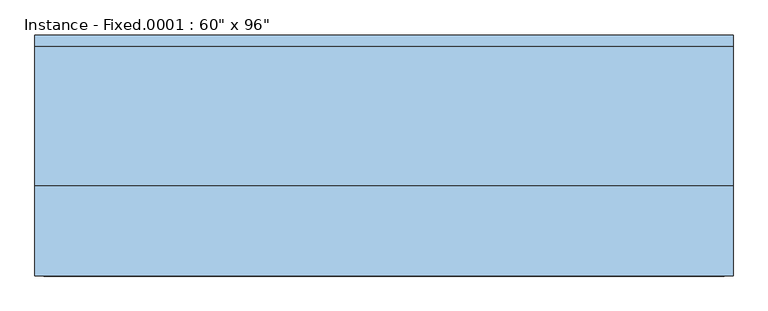
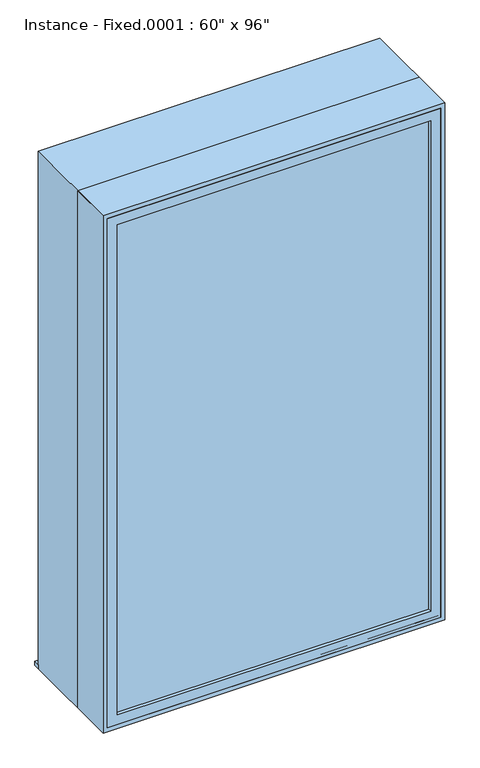
"""IFC4 building model written with IfcOpenShell, lengths in millimetres: window geometry."""

from ifc_helpers import new_model, si_unit, frame, origin, place, context, project, spatial, polyline, outline, extrude, source, transform, mapped, element, save


def window_e9f06afb(model_context):
    return source(origin(), model_context, "Body", "SweptSolid", [
        extrude(outline(polyline([(-800.1, 177.8), (723.9, 177.8), (723.9, 152.4), (-800.1, 152.4), (-800.1, 177.8)])), frame((0.0, 0.0, 609.6), z_axis=(0.0, 0.0, 1.0), x_axis=(1.0, 0.0, 0.0)), (0.0, 0.0, 1.0), 19.05),
        extrude(outline(polyline([(660.4, -333.375), (-736.6, -333.375), (-736.6, -320.675), (660.4, -320.675), (660.4, -333.375)])), frame((0.0, 0.0, 673.1), z_axis=(0.0, 0.0, 1.0), x_axis=(1.0, 0.0, 0.0)), (0.0, 0.0, 1.0), 2311.4),
        extrude(outline(polyline([(3028.95, -781.05), (628.65, -781.05), (628.65, 704.85), (3028.95, 704.85), (3028.95, -781.05)]), holes=[polyline([(2984.5, -736.6), (2984.5, 660.4), (673.1, 660.4), (673.1, -736.6), (2984.5, -736.6)])]), frame((0.0, -349.25, 0.0), z_axis=(0.0, 1.0, 0.0), x_axis=(0.0, 0.0, 1.0)), (0.0, 0.0, 1.0), 44.45),
        extrude(outline(polyline([(3048.0, -800.1), (609.6, -800.1), (609.6, 723.9), (3048.0, 723.9), (3048.0, -800.1)]), holes=[polyline([(3016.25, -768.35), (3016.25, 692.15), (641.35, 692.15), (641.35, -768.35), (3016.25, -768.35)])]), frame((0.0, -349.25, 0.0), z_axis=(0.0, 1.0, 0.0), x_axis=(0.0, 0.0, 1.0)), (0.0, 0.0, 1.0), 196.85),
        extrude(outline(polyline([(3048.0, 723.9), (3048.0, -800.1), (609.6, -800.1), (609.6, 723.9), (3048.0, 723.9)]), holes=[polyline([(3028.95, 704.85), (628.65, 704.85), (628.65, -781.05), (3028.95, -781.05), (3028.95, 704.85)])]), frame((0.0, -349.25, 0.0), z_axis=(0.0, 1.0, 0.0), x_axis=(0.0, 0.0, 1.0)), (0.0, 0.0, 1.0), 501.65),
    ])


if __name__ == "__main__":
    model = new_model("IFC4")
    model_context = context("Model", 3, world=origin())
    ifc_project = project(units=[si_unit("LENGTHUNIT", "METRE", prefix="MILLI")], contexts=[model_context])
    site = spatial("IfcSite", under=ifc_project)
    building = spatial("IfcBuilding", under=site)
    placement = place(None, origin())
    window_shape = window_e9f06afb(model_context)
    element("IfcWindow", 1, ObjectType="Instance - Fixed.0001 : 60\" x 96\"", at=placement, inside=building, context=model_context, shape_type="MappedRepresentation", body=[
        mapped(window_shape, transform((0.0, 0.0, 0.0), x_axis=(1.0, 0.0, 0.0), y_axis=(0.0, 1.0, 0.0), z_axis=(0.0, 0.0, 1.0))),
    ])
    save(model, "model.ifc")

# Revit data of these elements
# Type "Instance - Fixed.0001 : 60\" x 96\""
#   Type Mark = "13"
#   Construction Type Id = "MDOOR"
#   Assembly Code = "B2020100"
#   Analytic Construction = "Metal"
#   Heat Transfer Coefficient (U) = 0.651978 BTU/(h·ft²·°F)
#   Height [instance default] = 6' - 0"
#   Default Sill Height = 2' - 0"
#   Width [instance default] = 3' - 0"
#   Window Inset = 1' - 6"
#   Define Thermal Properties by = 1
#   Glass Pane Material = Glass
#   Sash Material = Door - Frame
#   Visual Light Transmittance = 0
#   Thermal Resistance (R) = 0
#   Solar Heat Gain Coefficient = 0
#   Wall Closure = (empty or 0)
# Element 1 (IfcWindow, "Instance - Fixed.0001 : 60\" x 96\"")
#   Height = 8' - 0"
#   Width = 5' - 0"
#   Materials on its faces: "Door - Frame", "Glass"
# Materials
#   "Glass": class "Glass", colour RGB 0 128 192, transparency 0.75, Description = "Soda Lime Glass", Cost = 0
#   "Door - Frame": colour RGB 118 70 51, transparency 0, Cost = 0
